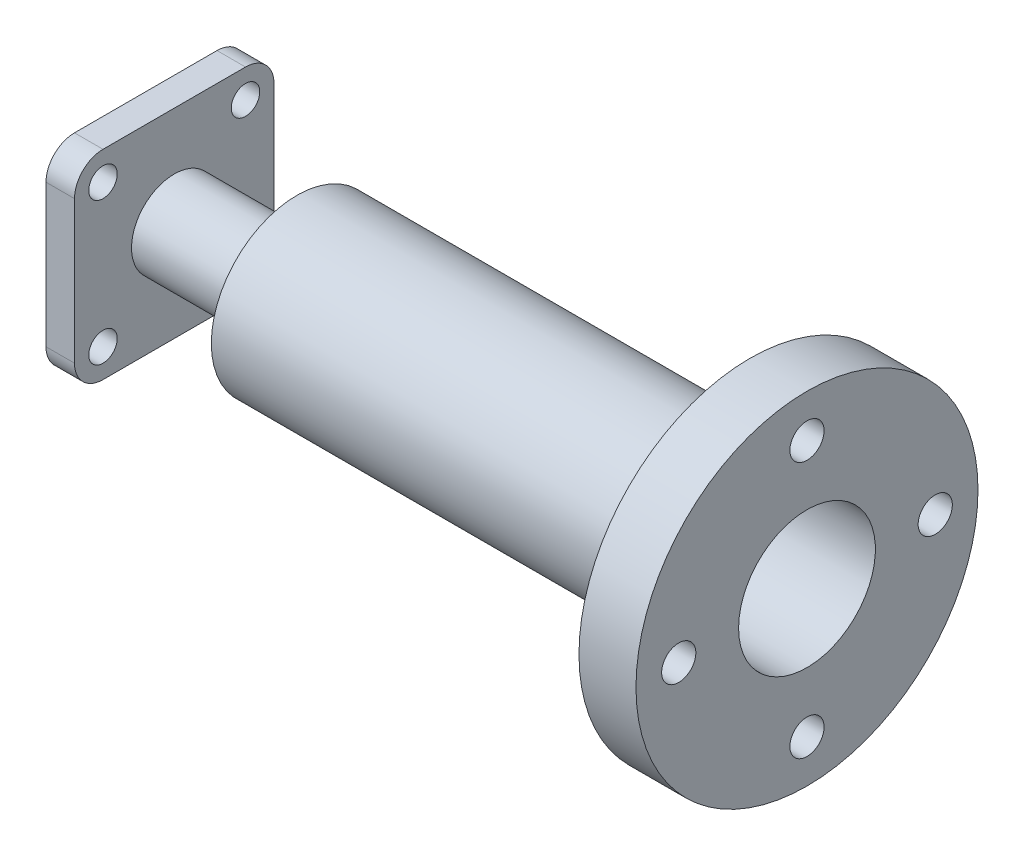
ISO-10303-21;
HEADER;
FILE_DESCRIPTION(('STEP AP214'),'2;1');
FILE_NAME('part.step','',(''),(''),'','','');
FILE_SCHEMA(('AUTOMOTIVE_DESIGN { 1 0 10303 214 1 1 1 1 }'));
ENDSEC;
DATA;
#1=APPLICATION_CONTEXT('core data for automotive mechanical design processes');
#2=APPLICATION_PROTOCOL_DEFINITION('international standard','automotive_design',2000,#1);
#3=PRODUCT_CONTEXT('',#1,'mechanical');
#4=PRODUCT('Part','Part','',(#3));
#5=PRODUCT_RELATED_PRODUCT_CATEGORY('part','',(#4));
#6=PRODUCT_DEFINITION_FORMATION('','',#4);
#7=PRODUCT_DEFINITION_CONTEXT('part definition',#1,'design');
#8=PRODUCT_DEFINITION('design','',#6,#7);
#9=PRODUCT_DEFINITION_SHAPE('','',#8);
#10=(LENGTH_UNIT() NAMED_UNIT(*) SI_UNIT(.MILLI.,.METRE.));
#11=(NAMED_UNIT(*) PLANE_ANGLE_UNIT() SI_UNIT($,.RADIAN.));
#12=(NAMED_UNIT(*) SI_UNIT($,.STERADIAN.) SOLID_ANGLE_UNIT());
#13=UNCERTAINTY_MEASURE_WITH_UNIT(LENGTH_MEASURE(1.E-05),#10,'distance_accuracy_value','');
#14=(GEOMETRIC_REPRESENTATION_CONTEXT(3) GLOBAL_UNCERTAINTY_ASSIGNED_CONTEXT((#13)) GLOBAL_UNIT_ASSIGNED_CONTEXT((#10,
#11,#12)) REPRESENTATION_CONTEXT('',''));
#15=CARTESIAN_POINT('',(0.,0.,0.));
#16=DIRECTION('',(0.,0.,1.));
#17=DIRECTION('',(1.,0.,0.));
#18=AXIS2_PLACEMENT_3D('',#15,#16,#17);
#19=CARTESIAN_POINT('',(0.,0.,0.));
#20=DIRECTION('',(-1.,0.,0.));
#21=DIRECTION('',(0.,0.,1.));
#22=AXIS2_PLACEMENT_3D('',#19,#20,#21);
#23=CYLINDRICAL_SURFACE('',#22,15.);
#24=CARTESIAN_POINT('',(0.,0.,0.));
#25=DIRECTION('',(-1.,0.,0.));
#26=DIRECTION('',(0.,0.,1.));
#27=AXIS2_PLACEMENT_3D('',#24,#25,#26);
#28=CIRCLE('',#27,15.);
#29=CARTESIAN_POINT('',(0.,0.,15.));
#30=VERTEX_POINT('',#29);
#31=EDGE_CURVE('E170',#30,#30,#28,.T.);
#32=ORIENTED_EDGE('',*,*,#31,.F.);
#33=EDGE_LOOP('',(#32));
#34=FACE_BOUND('',#33,.T.);
#35=CARTESIAN_POINT('',(43.,0.,0.));
#36=DIRECTION('',(-1.,0.,0.));
#37=DIRECTION('',(0.,0.,1.));
#38=AXIS2_PLACEMENT_3D('',#35,#36,#37);
#39=CIRCLE('',#38,15.);
#40=CARTESIAN_POINT('',(43.,0.,15.));
#41=VERTEX_POINT('',#40);
#42=EDGE_CURVE('E163',#41,#41,#39,.T.);
#43=ORIENTED_EDGE('',*,*,#42,.T.);
#44=EDGE_LOOP('',(#43));
#45=FACE_BOUND('',#44,.T.);
#46=ADVANCED_FACE('F39',(#34,#45),#23,.T.);
#47=CARTESIAN_POINT('',(43.,15.,0.));
#48=DIRECTION('',(1.,0.,0.));
#49=DIRECTION('',(0.,0.,-1.));
#50=AXIS2_PLACEMENT_3D('',#47,#48,#49);
#51=PLANE('',#50);
#52=ORIENTED_EDGE('',*,*,#42,.F.);
#53=EDGE_LOOP('',(#52));
#54=FACE_BOUND('',#53,.T.);
#55=CARTESIAN_POINT('',(43.,0.,0.));
#56=DIRECTION('',(-1.,0.,0.));
#57=DIRECTION('',(0.,0.,1.));
#58=AXIS2_PLACEMENT_3D('',#55,#56,#57);
#59=CIRCLE('',#58,30.);
#60=CARTESIAN_POINT('',(43.,0.,30.));
#61=VERTEX_POINT('',#60);
#62=EDGE_CURVE('E161',#61,#61,#59,.T.);
#63=ORIENTED_EDGE('',*,*,#62,.T.);
#64=EDGE_LOOP('',(#63));
#65=FACE_BOUND('',#64,.T.);
#66=ADVANCED_FACE('F330',(#54,#65),#51,.F.);
#67=CARTESIAN_POINT('',(0.,0.,0.));
#68=DIRECTION('',(-1.,0.,0.));
#69=DIRECTION('',(0.,0.,1.));
#70=AXIS2_PLACEMENT_3D('',#67,#68,#69);
#71=CYLINDRICAL_SURFACE('',#70,30.);
#72=ORIENTED_EDGE('',*,*,#62,.F.);
#73=EDGE_LOOP('',(#72));
#74=FACE_BOUND('',#73,.T.);
#75=CARTESIAN_POINT('',(202.,0.,0.));
#76=DIRECTION('',(-1.,0.,0.));
#77=DIRECTION('',(0.,0.,1.));
#78=AXIS2_PLACEMENT_3D('',#75,#76,#77);
#79=CIRCLE('',#78,30.);
#80=CARTESIAN_POINT('',(202.,0.,30.));
#81=VERTEX_POINT('',#80);
#82=EDGE_CURVE('E158',#81,#81,#79,.T.);
#83=ORIENTED_EDGE('',*,*,#82,.T.);
#84=EDGE_LOOP('',(#83));
#85=FACE_BOUND('',#84,.T.);
#86=ADVANCED_FACE('F267',(#74,#85),#71,.T.);
#87=CARTESIAN_POINT('',(202.,30.,0.));
#88=DIRECTION('',(1.,0.,0.));
#89=DIRECTION('',(0.,0.,-1.));
#90=AXIS2_PLACEMENT_3D('',#87,#88,#89);
#91=PLANE('',#90);
#92=CARTESIAN_POINT('',(202.,45.,-1.57116660247941E-13));
#93=DIRECTION('',(-1.,0.,0.));
#94=DIRECTION('',(0.,1.,0.));
#95=AXIS2_PLACEMENT_3D('',#92,#93,#94);
#96=CIRCLE('',#95,6.);
#97=CARTESIAN_POINT('',(202.,51.,-1.78065548281E-13));
#98=VERTEX_POINT('',#97);
#99=EDGE_CURVE('E246',#98,#98,#96,.T.);
#100=ORIENTED_EDGE('',*,*,#99,.F.);
#101=EDGE_LOOP('',(#100));
#102=FACE_BOUND('',#101,.T.);
#103=CARTESIAN_POINT('',(202.,0.,-45.));
#104=DIRECTION('',(-1.,0.,0.));
#105=DIRECTION('',(0.,0.,-1.));
#106=AXIS2_PLACEMENT_3D('',#103,#104,#105);
#107=CIRCLE('',#106,6.);
#108=CARTESIAN_POINT('',(202.,0.,-51.));
#109=VERTEX_POINT('',#108);
#110=EDGE_CURVE('E244',#109,#109,#107,.T.);
#111=ORIENTED_EDGE('',*,*,#110,.F.);
#112=EDGE_LOOP('',(#111));
#113=FACE_BOUND('',#112,.T.);
#114=CARTESIAN_POINT('',(202.,-45.,4.71349980743823E-13));
#115=DIRECTION('',(-1.,0.,0.));
#116=DIRECTION('',(0.,-1.,0.));
#117=AXIS2_PLACEMENT_3D('',#114,#115,#116);
#118=CIRCLE('',#117,6.);
#119=CARTESIAN_POINT('',(202.,-51.,5.34196644842999E-13));
#120=VERTEX_POINT('',#119);
#121=EDGE_CURVE('E240',#120,#120,#118,.T.);
#122=ORIENTED_EDGE('',*,*,#121,.F.);
#123=EDGE_LOOP('',(#122));
#124=FACE_BOUND('',#123,.T.);
#125=CARTESIAN_POINT('',(202.,0.,45.));
#126=DIRECTION('',(-1.,0.,0.));
#127=DIRECTION('',(0.,0.,1.));
#128=AXIS2_PLACEMENT_3D('',#125,#126,#127);
#129=CIRCLE('',#128,6.);
#130=CARTESIAN_POINT('',(202.,0.,51.));
#131=VERTEX_POINT('',#130);
#132=EDGE_CURVE('E232',#131,#131,#129,.T.);
#133=ORIENTED_EDGE('',*,*,#132,.F.);
#134=EDGE_LOOP('',(#133));
#135=FACE_BOUND('',#134,.T.);
#136=ORIENTED_EDGE('',*,*,#82,.F.);
#137=EDGE_LOOP('',(#136));
#138=FACE_BOUND('',#137,.T.);
#139=CARTESIAN_POINT('',(202.,0.,0.));
#140=DIRECTION('',(-1.,0.,0.));
#141=DIRECTION('',(0.,0.,1.));
#142=AXIS2_PLACEMENT_3D('',#139,#140,#141);
#143=CIRCLE('',#142,60.);
#144=CARTESIAN_POINT('',(202.,0.,60.));
#145=VERTEX_POINT('',#144);
#146=EDGE_CURVE('E154',#145,#145,#143,.T.);
#147=ORIENTED_EDGE('',*,*,#146,.T.);
#148=EDGE_LOOP('',(#147));
#149=FACE_BOUND('',#148,.T.);
#150=ADVANCED_FACE('F264',(#102,#113,#124,#135,#138,#149),#91,.F.);
#151=CARTESIAN_POINT('',(0.,0.,0.));
#152=DIRECTION('',(-1.,0.,0.));
#153=DIRECTION('',(0.,0.,1.));
#154=AXIS2_PLACEMENT_3D('',#151,#152,#153);
#155=CYLINDRICAL_SURFACE('',#154,60.);
#156=ORIENTED_EDGE('',*,*,#146,.F.);
#157=EDGE_LOOP('',(#156));
#158=FACE_BOUND('',#157,.T.);
#159=CARTESIAN_POINT('',(222.,0.,0.));
#160=DIRECTION('',(-1.,0.,0.));
#161=DIRECTION('',(0.,0.,1.));
#162=AXIS2_PLACEMENT_3D('',#159,#160,#161);
#163=CIRCLE('',#162,60.);
#164=CARTESIAN_POINT('',(222.,0.,60.));
#165=VERTEX_POINT('',#164);
#166=EDGE_CURVE('E155',#165,#165,#163,.T.);
#167=ORIENTED_EDGE('',*,*,#166,.T.);
#168=EDGE_LOOP('',(#167));
#169=FACE_BOUND('',#168,.T.);
#170=ADVANCED_FACE('F268',(#158,#169),#155,.T.);
#171=CARTESIAN_POINT('',(222.,60.,0.));
#172=DIRECTION('',(-1.,0.,0.));
#173=DIRECTION('',(0.,0.,1.));
#174=AXIS2_PLACEMENT_3D('',#171,#172,#173);
#175=PLANE('',#174);
#176=CARTESIAN_POINT('',(222.,45.,-1.57116660247941E-13));
#177=DIRECTION('',(-1.,0.,0.));
#178=DIRECTION('',(0.,1.,0.));
#179=AXIS2_PLACEMENT_3D('',#176,#177,#178);
#180=CIRCLE('',#179,6.);
#181=CARTESIAN_POINT('',(222.,51.,-1.78065548281E-13));
#182=VERTEX_POINT('',#181);
#183=EDGE_CURVE('E231',#182,#182,#180,.T.);
#184=ORIENTED_EDGE('',*,*,#183,.T.);
#185=EDGE_LOOP('',(#184));
#186=FACE_BOUND('',#185,.T.);
#187=CARTESIAN_POINT('',(222.,0.,-45.));
#188=DIRECTION('',(-1.,0.,0.));
#189=DIRECTION('',(0.,0.,-1.));
#190=AXIS2_PLACEMENT_3D('',#187,#188,#189);
#191=CIRCLE('',#190,6.);
#192=CARTESIAN_POINT('',(222.,0.,-51.));
#193=VERTEX_POINT('',#192);
#194=EDGE_CURVE('E247',#193,#193,#191,.T.);
#195=ORIENTED_EDGE('',*,*,#194,.T.);
#196=EDGE_LOOP('',(#195));
#197=FACE_BOUND('',#196,.T.);
#198=CARTESIAN_POINT('',(222.,-45.,4.71349980743823E-13));
#199=DIRECTION('',(-1.,0.,0.));
#200=DIRECTION('',(0.,-1.,0.));
#201=AXIS2_PLACEMENT_3D('',#198,#199,#200);
#202=CIRCLE('',#201,6.);
#203=CARTESIAN_POINT('',(222.,-51.,5.34196644842999E-13));
#204=VERTEX_POINT('',#203);
#205=EDGE_CURVE('E238',#204,#204,#202,.T.);
#206=ORIENTED_EDGE('',*,*,#205,.T.);
#207=EDGE_LOOP('',(#206));
#208=FACE_BOUND('',#207,.T.);
#209=CARTESIAN_POINT('',(222.,0.,45.));
#210=DIRECTION('',(-1.,0.,0.));
#211=DIRECTION('',(0.,0.,1.));
#212=AXIS2_PLACEMENT_3D('',#209,#210,#211);
#213=CIRCLE('',#212,6.);
#214=CARTESIAN_POINT('',(222.,0.,51.));
#215=VERTEX_POINT('',#214);
#216=EDGE_CURVE('E220',#215,#215,#213,.T.);
#217=ORIENTED_EDGE('',*,*,#216,.T.);
#218=EDGE_LOOP('',(#217));
#219=FACE_BOUND('',#218,.T.);
#220=ORIENTED_EDGE('',*,*,#166,.F.);
#221=EDGE_LOOP('',(#220));
#222=FACE_BOUND('',#221,.T.);
#223=CARTESIAN_POINT('',(222.,0.,0.));
#224=DIRECTION('',(-1.,0.,0.));
#225=DIRECTION('',(0.,0.,1.));
#226=AXIS2_PLACEMENT_3D('',#223,#224,#225);
#227=CIRCLE('',#226,24.);
#228=CARTESIAN_POINT('',(222.,0.,24.));
#229=VERTEX_POINT('',#228);
#230=EDGE_CURVE('E149',#229,#229,#227,.T.);
#231=ORIENTED_EDGE('',*,*,#230,.T.);
#232=EDGE_LOOP('',(#231));
#233=FACE_BOUND('',#232,.T.);
#234=ADVANCED_FACE('F254',(#186,#197,#208,#219,#222,#233),#175,.F.);
#235=CARTESIAN_POINT('',(0.,0.,0.));
#236=DIRECTION('',(-1.,0.,0.));
#237=DIRECTION('',(0.,0.,1.));
#238=AXIS2_PLACEMENT_3D('',#235,#236,#237);
#239=CYLINDRICAL_SURFACE('',#238,24.);
#240=ORIENTED_EDGE('',*,*,#230,.F.);
#241=EDGE_LOOP('',(#240));
#242=FACE_BOUND('',#241,.T.);
#243=CARTESIAN_POINT('',(49.,0.,0.));
#244=DIRECTION('',(-1.,0.,0.));
#245=DIRECTION('',(0.,0.,1.));
#246=AXIS2_PLACEMENT_3D('',#243,#244,#245);
#247=CIRCLE('',#246,24.);
#248=CARTESIAN_POINT('',(49.,0.,24.));
#249=VERTEX_POINT('',#248);
#250=EDGE_CURVE('E148',#249,#249,#247,.T.);
#251=ORIENTED_EDGE('',*,*,#250,.T.);
#252=EDGE_LOOP('',(#251));
#253=FACE_BOUND('',#252,.T.);
#254=ADVANCED_FACE('F289',(#242,#253),#239,.F.);
#255=CARTESIAN_POINT('',(49.,24.,0.));
#256=DIRECTION('',(-1.,0.,0.));
#257=DIRECTION('',(0.,0.,1.));
#258=AXIS2_PLACEMENT_3D('',#255,#256,#257);
#259=PLANE('',#258);
#260=ORIENTED_EDGE('',*,*,#250,.F.);
#261=EDGE_LOOP('',(#260));
#262=FACE_BOUND('',#261,.T.);
#263=CARTESIAN_POINT('',(49.,0.,0.));
#264=DIRECTION('',(-1.,0.,0.));
#265=DIRECTION('',(0.,0.,1.));
#266=AXIS2_PLACEMENT_3D('',#263,#264,#265);
#267=CIRCLE('',#266,9.00000000000001);
#268=CARTESIAN_POINT('',(49.,0.,9.00000000000001));
#269=VERTEX_POINT('',#268);
#270=EDGE_CURVE('E141',#269,#269,#267,.T.);
#271=ORIENTED_EDGE('',*,*,#270,.T.);
#272=EDGE_LOOP('',(#271));
#273=FACE_BOUND('',#272,.T.);
#274=ADVANCED_FACE('F294',(#262,#273),#259,.F.);
#275=CARTESIAN_POINT('',(0.,0.,0.));
#276=DIRECTION('',(-1.,0.,0.));
#277=DIRECTION('',(0.,0.,1.));
#278=AXIS2_PLACEMENT_3D('',#275,#276,#277);
#279=CYLINDRICAL_SURFACE('',#278,9.);
#280=ORIENTED_EDGE('',*,*,#270,.F.);
#281=EDGE_LOOP('',(#280));
#282=FACE_BOUND('',#281,.T.);
#283=CARTESIAN_POINT('',(0.,0.,0.));
#284=DIRECTION('',(-1.,0.,0.));
#285=DIRECTION('',(0.,0.,1.));
#286=AXIS2_PLACEMENT_3D('',#283,#284,#285);
#287=CIRCLE('',#286,9.);
#288=CARTESIAN_POINT('',(0.,0.,9.));
#289=VERTEX_POINT('',#288);
#290=EDGE_CURVE('E138',#289,#289,#287,.T.);
#291=ORIENTED_EDGE('',*,*,#290,.T.);
#292=EDGE_LOOP('',(#291));
#293=FACE_BOUND('',#292,.T.);
#294=ADVANCED_FACE('F300',(#282,#293),#279,.F.);
#295=CARTESIAN_POINT('',(0.,0.,0.));
#296=DIRECTION('',(-1.,0.,0.));
#297=DIRECTION('',(0.,0.,1.));
#298=AXIS2_PLACEMENT_3D('',#295,#296,#297);
#299=PLANE('',#298);
#300=CARTESIAN_POINT('',(0.,-25.,25.));
#301=DIRECTION('',(-1.,0.,0.));
#302=DIRECTION('',(0.,0.,1.));
#303=AXIS2_PLACEMENT_3D('',#300,#301,#302);
#304=CIRCLE('',#303,5.);
#305=CARTESIAN_POINT('',(0.,-25.,30.));
#306=VERTEX_POINT('',#305);
#307=EDGE_CURVE('E216',#306,#306,#304,.T.);
#308=ORIENTED_EDGE('',*,*,#307,.T.);
#309=EDGE_LOOP('',(#308));
#310=FACE_BOUND('',#309,.T.);
#311=CARTESIAN_POINT('',(0.,-25.,-25.));
#312=DIRECTION('',(-1.,0.,0.));
#313=DIRECTION('',(0.,0.,1.));
#314=AXIS2_PLACEMENT_3D('',#311,#312,#313);
#315=CIRCLE('',#314,5.);
#316=CARTESIAN_POINT('',(0.,-25.,-20.));
#317=VERTEX_POINT('',#316);
#318=EDGE_CURVE('E224',#317,#317,#315,.T.);
#319=ORIENTED_EDGE('',*,*,#318,.T.);
#320=EDGE_LOOP('',(#319));
#321=FACE_BOUND('',#320,.T.);
#322=CARTESIAN_POINT('',(0.,25.,-25.));
#323=DIRECTION('',(-1.,0.,0.));
#324=DIRECTION('',(0.,0.,1.));
#325=AXIS2_PLACEMENT_3D('',#322,#323,#324);
#326=CIRCLE('',#325,5.);
#327=CARTESIAN_POINT('',(0.,25.,-20.));
#328=VERTEX_POINT('',#327);
#329=EDGE_CURVE('E211',#328,#328,#326,.T.);
#330=ORIENTED_EDGE('',*,*,#329,.T.);
#331=EDGE_LOOP('',(#330));
#332=FACE_BOUND('',#331,.T.);
#333=CARTESIAN_POINT('',(0.,25.,25.));
#334=DIRECTION('',(-1.,0.,0.));
#335=DIRECTION('',(0.,0.,1.));
#336=AXIS2_PLACEMENT_3D('',#333,#334,#335);
#337=CIRCLE('',#336,5.);
#338=CARTESIAN_POINT('',(0.,25.,30.));
#339=VERTEX_POINT('',#338);
#340=EDGE_CURVE('E200',#339,#339,#337,.T.);
#341=ORIENTED_EDGE('',*,*,#340,.T.);
#342=EDGE_LOOP('',(#341));
#343=FACE_BOUND('',#342,.T.);
#344=ORIENTED_EDGE('',*,*,#31,.T.);
#345=EDGE_LOOP('',(#344));
#346=FACE_BOUND('',#345,.T.);
#347=DIRECTION('',(0.,0.,1.));
#348=VECTOR('',#347,1.);
#349=CARTESIAN_POINT('',(0.,-35.,-35.));
#350=LINE('',#349,#348);
#351=CARTESIAN_POINT('',(0.,-35.,-25.));
#352=VERTEX_POINT('',#351);
#353=CARTESIAN_POINT('',(0.,-35.,25.));
#354=VERTEX_POINT('',#353);
#355=EDGE_CURVE('E125',#352,#354,#350,.T.);
#356=ORIENTED_EDGE('',*,*,#355,.F.);
#357=CARTESIAN_POINT('',(0.,-25.,-25.));
#358=DIRECTION('',(-1.,0.,0.));
#359=DIRECTION('',(0.,0.,1.));
#360=AXIS2_PLACEMENT_3D('',#357,#358,#359);
#361=CIRCLE('',#360,10.);
#362=CARTESIAN_POINT('',(0.,-25.,-35.));
#363=VERTEX_POINT('',#362);
#364=EDGE_CURVE('E104',#352,#363,#361,.F.);
#365=ORIENTED_EDGE('',*,*,#364,.T.);
#366=DIRECTION('',(0.,-1.,0.));
#367=VECTOR('',#366,1.);
#368=CARTESIAN_POINT('',(0.,35.,-35.));
#369=LINE('',#368,#367);
#370=CARTESIAN_POINT('',(0.,25.,-35.));
#371=VERTEX_POINT('',#370);
#372=EDGE_CURVE('E132',#371,#363,#369,.T.);
#373=ORIENTED_EDGE('',*,*,#372,.F.);
#374=CARTESIAN_POINT('',(0.,25.,-25.));
#375=DIRECTION('',(-1.,0.,0.));
#376=DIRECTION('',(0.,0.,1.));
#377=AXIS2_PLACEMENT_3D('',#374,#375,#376);
#378=CIRCLE('',#377,10.);
#379=CARTESIAN_POINT('',(0.,35.,-25.));
#380=VERTEX_POINT('',#379);
#381=EDGE_CURVE('E127',#371,#380,#378,.F.);
#382=ORIENTED_EDGE('',*,*,#381,.T.);
#383=DIRECTION('',(0.,0.,-1.));
#384=VECTOR('',#383,1.);
#385=CARTESIAN_POINT('',(0.,35.,-35.));
#386=LINE('',#385,#384);
#387=CARTESIAN_POINT('',(0.,35.,25.));
#388=VERTEX_POINT('',#387);
#389=EDGE_CURVE('E137',#388,#380,#386,.T.);
#390=ORIENTED_EDGE('',*,*,#389,.F.);
#391=CARTESIAN_POINT('',(0.,25.,25.));
#392=DIRECTION('',(-1.,0.,0.));
#393=DIRECTION('',(0.,0.,1.));
#394=AXIS2_PLACEMENT_3D('',#391,#392,#393);
#395=CIRCLE('',#394,10.);
#396=CARTESIAN_POINT('',(0.,25.,35.));
#397=VERTEX_POINT('',#396);
#398=EDGE_CURVE('E172',#388,#397,#395,.F.);
#399=ORIENTED_EDGE('',*,*,#398,.T.);
#400=DIRECTION('',(0.,1.,0.));
#401=VECTOR('',#400,1.);
#402=CARTESIAN_POINT('',(0.,35.,35.));
#403=LINE('',#402,#401);
#404=CARTESIAN_POINT('',(0.,-25.,35.));
#405=VERTEX_POINT('',#404);
#406=EDGE_CURVE('E191',#405,#397,#403,.T.);
#407=ORIENTED_EDGE('',*,*,#406,.F.);
#408=CARTESIAN_POINT('',(0.,-25.,25.));
#409=DIRECTION('',(-1.,0.,0.));
#410=DIRECTION('',(0.,0.,1.));
#411=AXIS2_PLACEMENT_3D('',#408,#409,#410);
#412=CIRCLE('',#411,10.);
#413=EDGE_CURVE('E116',#405,#354,#412,.F.);
#414=ORIENTED_EDGE('',*,*,#413,.T.);
#415=EDGE_LOOP('',(#356,#365,#373,#382,#390,#399,#407,#414));
#416=FACE_BOUND('',#415,.T.);
#417=ADVANCED_FACE('F129',(#310,#321,#332,#343,#346,#416),#299,.F.);
#418=CARTESIAN_POINT('',(-10.,0.,0.));
#419=DIRECTION('',(-1.,0.,0.));
#420=DIRECTION('',(0.,0.,1.));
#421=AXIS2_PLACEMENT_3D('',#418,#419,#420);
#422=PLANE('',#421);
#423=CARTESIAN_POINT('',(-10.,-25.,25.));
#424=DIRECTION('',(-1.,0.,0.));
#425=DIRECTION('',(0.,0.,1.));
#426=AXIS2_PLACEMENT_3D('',#423,#424,#425);
#427=CIRCLE('',#426,5.);
#428=CARTESIAN_POINT('',(-10.,-25.,30.));
#429=VERTEX_POINT('',#428);
#430=EDGE_CURVE('E213',#429,#429,#427,.T.);
#431=ORIENTED_EDGE('',*,*,#430,.F.);
#432=EDGE_LOOP('',(#431));
#433=FACE_BOUND('',#432,.T.);
#434=CARTESIAN_POINT('',(-10.,-25.,-25.));
#435=DIRECTION('',(-1.,0.,0.));
#436=DIRECTION('',(0.,0.,1.));
#437=AXIS2_PLACEMENT_3D('',#434,#435,#436);
#438=CIRCLE('',#437,5.);
#439=CARTESIAN_POINT('',(-10.,-25.,-20.));
#440=VERTEX_POINT('',#439);
#441=EDGE_CURVE('E219',#440,#440,#438,.T.);
#442=ORIENTED_EDGE('',*,*,#441,.F.);
#443=EDGE_LOOP('',(#442));
#444=FACE_BOUND('',#443,.T.);
#445=CARTESIAN_POINT('',(-10.,25.,-25.));
#446=DIRECTION('',(-1.,0.,0.));
#447=DIRECTION('',(0.,0.,1.));
#448=AXIS2_PLACEMENT_3D('',#445,#446,#447);
#449=CIRCLE('',#448,5.);
#450=CARTESIAN_POINT('',(-10.,25.,-20.));
#451=VERTEX_POINT('',#450);
#452=EDGE_CURVE('E226',#451,#451,#449,.T.);
#453=ORIENTED_EDGE('',*,*,#452,.F.);
#454=EDGE_LOOP('',(#453));
#455=FACE_BOUND('',#454,.T.);
#456=CARTESIAN_POINT('',(-10.,25.,25.));
#457=DIRECTION('',(-1.,0.,0.));
#458=DIRECTION('',(0.,0.,1.));
#459=AXIS2_PLACEMENT_3D('',#456,#457,#458);
#460=CIRCLE('',#459,5.);
#461=CARTESIAN_POINT('',(-10.,25.,30.));
#462=VERTEX_POINT('',#461);
#463=EDGE_CURVE('E205',#462,#462,#460,.T.);
#464=ORIENTED_EDGE('',*,*,#463,.F.);
#465=EDGE_LOOP('',(#464));
#466=FACE_BOUND('',#465,.T.);
#467=DIRECTION('',(0.,-1.,0.));
#468=VECTOR('',#467,1.);
#469=CARTESIAN_POINT('',(-10.,35.,-35.));
#470=LINE('',#469,#468);
#471=CARTESIAN_POINT('',(-10.,25.,-35.));
#472=VERTEX_POINT('',#471);
#473=CARTESIAN_POINT('',(-10.,-25.,-35.));
#474=VERTEX_POINT('',#473);
#475=EDGE_CURVE('E206',#472,#474,#470,.T.);
#476=ORIENTED_EDGE('',*,*,#475,.T.);
#477=CARTESIAN_POINT('',(-10.,-25.,-25.));
#478=DIRECTION('',(-1.,0.,0.));
#479=DIRECTION('',(0.,0.,1.));
#480=AXIS2_PLACEMENT_3D('',#477,#478,#479);
#481=CIRCLE('',#480,10.);
#482=CARTESIAN_POINT('',(-10.,-35.,-25.));
#483=VERTEX_POINT('',#482);
#484=EDGE_CURVE('E181',#474,#483,#481,.T.);
#485=ORIENTED_EDGE('',*,*,#484,.T.);
#486=DIRECTION('',(0.,0.,1.));
#487=VECTOR('',#486,1.);
#488=CARTESIAN_POINT('',(-10.,-35.,-35.));
#489=LINE('',#488,#487);
#490=CARTESIAN_POINT('',(-10.,-35.,25.));
#491=VERTEX_POINT('',#490);
#492=EDGE_CURVE('E123',#483,#491,#489,.T.);
#493=ORIENTED_EDGE('',*,*,#492,.T.);
#494=CARTESIAN_POINT('',(-10.,-25.,25.));
#495=DIRECTION('',(-1.,0.,0.));
#496=DIRECTION('',(0.,0.,1.));
#497=AXIS2_PLACEMENT_3D('',#494,#495,#496);
#498=CIRCLE('',#497,10.);
#499=CARTESIAN_POINT('',(-10.,-25.,35.));
#500=VERTEX_POINT('',#499);
#501=EDGE_CURVE('E182',#491,#500,#498,.T.);
#502=ORIENTED_EDGE('',*,*,#501,.T.);
#503=DIRECTION('',(0.,1.,0.));
#504=VECTOR('',#503,1.);
#505=CARTESIAN_POINT('',(-10.,35.,35.));
#506=LINE('',#505,#504);
#507=CARTESIAN_POINT('',(-10.,25.,35.));
#508=VERTEX_POINT('',#507);
#509=EDGE_CURVE('E131',#500,#508,#506,.T.);
#510=ORIENTED_EDGE('',*,*,#509,.T.);
#511=CARTESIAN_POINT('',(-10.,25.,25.));
#512=DIRECTION('',(-1.,0.,0.));
#513=DIRECTION('',(0.,0.,1.));
#514=AXIS2_PLACEMENT_3D('',#511,#512,#513);
#515=CIRCLE('',#514,10.);
#516=CARTESIAN_POINT('',(-10.,35.,25.));
#517=VERTEX_POINT('',#516);
#518=EDGE_CURVE('E58',#508,#517,#515,.T.);
#519=ORIENTED_EDGE('',*,*,#518,.T.);
#520=DIRECTION('',(0.,0.,-1.));
#521=VECTOR('',#520,1.);
#522=CARTESIAN_POINT('',(-10.,35.,-35.));
#523=LINE('',#522,#521);
#524=CARTESIAN_POINT('',(-10.,35.,-25.));
#525=VERTEX_POINT('',#524);
#526=EDGE_CURVE('E133',#517,#525,#523,.T.);
#527=ORIENTED_EDGE('',*,*,#526,.T.);
#528=CARTESIAN_POINT('',(-10.,25.,-25.));
#529=DIRECTION('',(-1.,0.,0.));
#530=DIRECTION('',(0.,0.,1.));
#531=AXIS2_PLACEMENT_3D('',#528,#529,#530);
#532=CIRCLE('',#531,10.);
#533=EDGE_CURVE('E179',#525,#472,#532,.T.);
#534=ORIENTED_EDGE('',*,*,#533,.T.);
#535=EDGE_LOOP('',(#476,#485,#493,#502,#510,#519,#527,#534));
#536=FACE_BOUND('',#535,.T.);
#537=ADVANCED_FACE('F322',(#433,#444,#455,#466,#536),#422,.T.);
#538=CARTESIAN_POINT('',(-10.,-35.,-35.));
#539=DIRECTION('',(0.,1.,0.));
#540=DIRECTION('',(0.,0.,1.));
#541=AXIS2_PLACEMENT_3D('',#538,#539,#540);
#542=PLANE('',#541);
#543=ORIENTED_EDGE('',*,*,#492,.F.);
#544=DIRECTION('',(1.,0.,0.));
#545=VECTOR('',#544,1.);
#546=CARTESIAN_POINT('',(-10.,-35.,-25.));
#547=LINE('',#546,#545);
#548=EDGE_CURVE('E108',#483,#352,#547,.T.);
#549=ORIENTED_EDGE('',*,*,#548,.T.);
#550=ORIENTED_EDGE('',*,*,#355,.T.);
#551=DIRECTION('',(1.,0.,0.));
#552=VECTOR('',#551,1.);
#553=CARTESIAN_POINT('',(-10.,-35.,25.));
#554=LINE('',#553,#552);
#555=EDGE_CURVE('E130',#354,#491,#554,.F.);
#556=ORIENTED_EDGE('',*,*,#555,.T.);
#557=EDGE_LOOP('',(#543,#549,#550,#556));
#558=FACE_BOUND('',#557,.T.);
#559=ADVANCED_FACE('F122',(#558),#542,.F.);
#560=CARTESIAN_POINT('',(-10.,35.,-35.));
#561=DIRECTION('',(0.,0.,1.));
#562=DIRECTION('',(0.,-1.,0.));
#563=AXIS2_PLACEMENT_3D('',#560,#561,#562);
#564=PLANE('',#563);
#565=ORIENTED_EDGE('',*,*,#372,.T.);
#566=DIRECTION('',(1.,0.,0.));
#567=VECTOR('',#566,1.);
#568=CARTESIAN_POINT('',(-10.,-25.,-35.));
#569=LINE('',#568,#567);
#570=EDGE_CURVE('E109',#363,#474,#569,.F.);
#571=ORIENTED_EDGE('',*,*,#570,.T.);
#572=ORIENTED_EDGE('',*,*,#475,.F.);
#573=DIRECTION('',(1.,0.,0.));
#574=VECTOR('',#573,1.);
#575=CARTESIAN_POINT('',(-10.,25.,-35.));
#576=LINE('',#575,#574);
#577=EDGE_CURVE('E113',#472,#371,#576,.T.);
#578=ORIENTED_EDGE('',*,*,#577,.T.);
#579=EDGE_LOOP('',(#565,#571,#572,#578));
#580=FACE_BOUND('',#579,.T.);
#581=ADVANCED_FACE('F354',(#580),#564,.F.);
#582=CARTESIAN_POINT('',(-10.,35.,-35.));
#583=DIRECTION('',(0.,-1.,0.));
#584=DIRECTION('',(0.,0.,-1.));
#585=AXIS2_PLACEMENT_3D('',#582,#583,#584);
#586=PLANE('',#585);
#587=ORIENTED_EDGE('',*,*,#526,.F.);
#588=DIRECTION('',(1.,0.,0.));
#589=VECTOR('',#588,1.);
#590=CARTESIAN_POINT('',(-10.,35.,25.));
#591=LINE('',#590,#589);
#592=EDGE_CURVE('E11',#517,#388,#591,.T.);
#593=ORIENTED_EDGE('',*,*,#592,.T.);
#594=ORIENTED_EDGE('',*,*,#389,.T.);
#595=DIRECTION('',(1.,0.,0.));
#596=VECTOR('',#595,1.);
#597=CARTESIAN_POINT('',(-10.,35.,-25.));
#598=LINE('',#597,#596);
#599=EDGE_CURVE('E50',#380,#525,#598,.F.);
#600=ORIENTED_EDGE('',*,*,#599,.T.);
#601=EDGE_LOOP('',(#587,#593,#594,#600));
#602=FACE_BOUND('',#601,.T.);
#603=ADVANCED_FACE('F317',(#602),#586,.F.);
#604=CARTESIAN_POINT('',(-10.,35.,35.));
#605=DIRECTION('',(0.,0.,-1.));
#606=DIRECTION('',(0.,1.,0.));
#607=AXIS2_PLACEMENT_3D('',#604,#605,#606);
#608=PLANE('',#607);
#609=ORIENTED_EDGE('',*,*,#509,.F.);
#610=DIRECTION('',(1.,0.,0.));
#611=VECTOR('',#610,1.);
#612=CARTESIAN_POINT('',(-10.,-25.,35.));
#613=LINE('',#612,#611);
#614=EDGE_CURVE('E187',#500,#405,#613,.T.);
#615=ORIENTED_EDGE('',*,*,#614,.T.);
#616=ORIENTED_EDGE('',*,*,#406,.T.);
#617=DIRECTION('',(1.,0.,0.));
#618=VECTOR('',#617,1.);
#619=CARTESIAN_POINT('',(-10.,25.,35.));
#620=LINE('',#619,#618);
#621=EDGE_CURVE('E183',#397,#508,#620,.F.);
#622=ORIENTED_EDGE('',*,*,#621,.T.);
#623=EDGE_LOOP('',(#609,#615,#616,#622));
#624=FACE_BOUND('',#623,.T.);
#625=ADVANCED_FACE('F194',(#624),#608,.F.);
#626=ORIENTED_EDGE('',*,*,#290,.F.);
#627=EDGE_LOOP('',(#626));
#628=FACE_BOUND('',#627,.T.);
#629=ADVANCED_FACE('F310',(#628),#299,.F.);
#630=CARTESIAN_POINT('',(-10.,-25.,-25.));
#631=DIRECTION('',(1.,0.,0.));
#632=DIRECTION('',(0.,0.,-1.));
#633=AXIS2_PLACEMENT_3D('',#630,#631,#632);
#634=CYLINDRICAL_SURFACE('',#633,10.);
#635=ORIENTED_EDGE('',*,*,#484,.F.);
#636=ORIENTED_EDGE('',*,*,#570,.F.);
#637=ORIENTED_EDGE('',*,*,#364,.F.);
#638=ORIENTED_EDGE('',*,*,#548,.F.);
#639=EDGE_LOOP('',(#635,#636,#637,#638));
#640=FACE_BOUND('',#639,.T.);
#641=ADVANCED_FACE('F107',(#640),#634,.T.);
#642=CARTESIAN_POINT('',(-10.,-25.,25.));
#643=DIRECTION('',(1.,0.,0.));
#644=DIRECTION('',(0.,0.,-1.));
#645=AXIS2_PLACEMENT_3D('',#642,#643,#644);
#646=CYLINDRICAL_SURFACE('',#645,10.);
#647=ORIENTED_EDGE('',*,*,#501,.F.);
#648=ORIENTED_EDGE('',*,*,#555,.F.);
#649=ORIENTED_EDGE('',*,*,#413,.F.);
#650=ORIENTED_EDGE('',*,*,#614,.F.);
#651=EDGE_LOOP('',(#647,#648,#649,#650));
#652=FACE_BOUND('',#651,.T.);
#653=ADVANCED_FACE('F316',(#652),#646,.T.);
#654=CARTESIAN_POINT('',(-10.,25.,25.));
#655=DIRECTION('',(1.,0.,0.));
#656=DIRECTION('',(0.,0.,-1.));
#657=AXIS2_PLACEMENT_3D('',#654,#655,#656);
#658=CYLINDRICAL_SURFACE('',#657,10.);
#659=ORIENTED_EDGE('',*,*,#518,.F.);
#660=ORIENTED_EDGE('',*,*,#621,.F.);
#661=ORIENTED_EDGE('',*,*,#398,.F.);
#662=ORIENTED_EDGE('',*,*,#592,.F.);
#663=EDGE_LOOP('',(#659,#660,#661,#662));
#664=FACE_BOUND('',#663,.T.);
#665=ADVANCED_FACE('F340',(#664),#658,.T.);
#666=CARTESIAN_POINT('',(-10.,25.,-25.));
#667=DIRECTION('',(1.,0.,0.));
#668=DIRECTION('',(0.,0.,-1.));
#669=AXIS2_PLACEMENT_3D('',#666,#667,#668);
#670=CYLINDRICAL_SURFACE('',#669,10.);
#671=ORIENTED_EDGE('',*,*,#533,.F.);
#672=ORIENTED_EDGE('',*,*,#599,.F.);
#673=ORIENTED_EDGE('',*,*,#381,.F.);
#674=ORIENTED_EDGE('',*,*,#577,.F.);
#675=EDGE_LOOP('',(#671,#672,#673,#674));
#676=FACE_BOUND('',#675,.T.);
#677=ADVANCED_FACE('F41',(#676),#670,.T.);
#678=CARTESIAN_POINT('',(0.,25.,25.));
#679=DIRECTION('',(-1.,0.,0.));
#680=DIRECTION('',(0.,0.,1.));
#681=AXIS2_PLACEMENT_3D('',#678,#679,#680);
#682=CYLINDRICAL_SURFACE('',#681,5.);
#683=ORIENTED_EDGE('',*,*,#340,.F.);
#684=EDGE_LOOP('',(#683));
#685=FACE_BOUND('',#684,.T.);
#686=ORIENTED_EDGE('',*,*,#463,.T.);
#687=EDGE_LOOP('',(#686));
#688=FACE_BOUND('',#687,.T.);
#689=ADVANCED_FACE('F347',(#685,#688),#682,.F.);
#690=CARTESIAN_POINT('',(0.,25.,-25.));
#691=DIRECTION('',(-1.,0.,0.));
#692=DIRECTION('',(0.,0.,1.));
#693=AXIS2_PLACEMENT_3D('',#690,#691,#692);
#694=CYLINDRICAL_SURFACE('',#693,5.);
#695=ORIENTED_EDGE('',*,*,#329,.F.);
#696=EDGE_LOOP('',(#695));
#697=FACE_BOUND('',#696,.T.);
#698=ORIENTED_EDGE('',*,*,#452,.T.);
#699=EDGE_LOOP('',(#698));
#700=FACE_BOUND('',#699,.T.);
#701=ADVANCED_FACE('F361',(#697,#700),#694,.F.);
#702=CARTESIAN_POINT('',(0.,-25.,-25.));
#703=DIRECTION('',(-1.,0.,0.));
#704=DIRECTION('',(0.,0.,1.));
#705=AXIS2_PLACEMENT_3D('',#702,#703,#704);
#706=CYLINDRICAL_SURFACE('',#705,5.);
#707=ORIENTED_EDGE('',*,*,#318,.F.);
#708=EDGE_LOOP('',(#707));
#709=FACE_BOUND('',#708,.T.);
#710=ORIENTED_EDGE('',*,*,#441,.T.);
#711=EDGE_LOOP('',(#710));
#712=FACE_BOUND('',#711,.T.);
#713=ADVANCED_FACE('F369',(#709,#712),#706,.F.);
#714=CARTESIAN_POINT('',(0.,-25.,25.));
#715=DIRECTION('',(-1.,0.,0.));
#716=DIRECTION('',(0.,0.,1.));
#717=AXIS2_PLACEMENT_3D('',#714,#715,#716);
#718=CYLINDRICAL_SURFACE('',#717,5.);
#719=ORIENTED_EDGE('',*,*,#307,.F.);
#720=EDGE_LOOP('',(#719));
#721=FACE_BOUND('',#720,.T.);
#722=ORIENTED_EDGE('',*,*,#430,.T.);
#723=EDGE_LOOP('',(#722));
#724=FACE_BOUND('',#723,.T.);
#725=ADVANCED_FACE('F364',(#721,#724),#718,.F.);
#726=CARTESIAN_POINT('',(222.,0.,45.));
#727=DIRECTION('',(-1.,0.,0.));
#728=DIRECTION('',(0.,0.,1.));
#729=AXIS2_PLACEMENT_3D('',#726,#727,#728);
#730=CYLINDRICAL_SURFACE('',#729,6.);
#731=ORIENTED_EDGE('',*,*,#216,.F.);
#732=EDGE_LOOP('',(#731));
#733=FACE_BOUND('',#732,.T.);
#734=ORIENTED_EDGE('',*,*,#132,.T.);
#735=EDGE_LOOP('',(#734));
#736=FACE_BOUND('',#735,.T.);
#737=ADVANCED_FACE('F366',(#733,#736),#730,.F.);
#738=CARTESIAN_POINT('',(222.,-45.,4.71349980743823E-13));
#739=DIRECTION('',(-1.,0.,0.));
#740=DIRECTION('',(0.,0.,1.));
#741=AXIS2_PLACEMENT_3D('',#738,#739,#740);
#742=CYLINDRICAL_SURFACE('',#741,6.);
#743=ORIENTED_EDGE('',*,*,#205,.F.);
#744=EDGE_LOOP('',(#743));
#745=FACE_BOUND('',#744,.T.);
#746=ORIENTED_EDGE('',*,*,#121,.T.);
#747=EDGE_LOOP('',(#746));
#748=FACE_BOUND('',#747,.T.);
#749=ADVANCED_FACE('F377',(#745,#748),#742,.F.);
#750=CARTESIAN_POINT('',(222.,0.,-45.));
#751=DIRECTION('',(-1.,0.,0.));
#752=DIRECTION('',(0.,0.,1.));
#753=AXIS2_PLACEMENT_3D('',#750,#751,#752);
#754=CYLINDRICAL_SURFACE('',#753,6.);
#755=ORIENTED_EDGE('',*,*,#194,.F.);
#756=EDGE_LOOP('',(#755));
#757=FACE_BOUND('',#756,.T.);
#758=ORIENTED_EDGE('',*,*,#110,.T.);
#759=EDGE_LOOP('',(#758));
#760=FACE_BOUND('',#759,.T.);
#761=ADVANCED_FACE('F261',(#757,#760),#754,.F.);
#762=CARTESIAN_POINT('',(222.,45.,-1.57116660247941E-13));
#763=DIRECTION('',(-1.,0.,0.));
#764=DIRECTION('',(0.,0.,1.));
#765=AXIS2_PLACEMENT_3D('',#762,#763,#764);
#766=CYLINDRICAL_SURFACE('',#765,6.);
#767=ORIENTED_EDGE('',*,*,#183,.F.);
#768=EDGE_LOOP('',(#767));
#769=FACE_BOUND('',#768,.T.);
#770=ORIENTED_EDGE('',*,*,#99,.T.);
#771=EDGE_LOOP('',(#770));
#772=FACE_BOUND('',#771,.T.);
#773=ADVANCED_FACE('F256',(#769,#772),#766,.F.);
#774=CLOSED_SHELL('',(#46,#66,#86,#150,#170,#234,#254,#274,#294,#417,#537,#559,#581,#603,#625,
#629,#641,#653,#665,#677,#689,#701,#713,#725,#737,#749,#761,#773));
#775=MANIFOLD_SOLID_BREP('B2',#774);
#776=ADVANCED_BREP_SHAPE_REPRESENTATION('',(#18,#775),#14);
#777=SHAPE_DEFINITION_REPRESENTATION(#9,#776);
ENDSEC;
END-ISO-10303-21;
